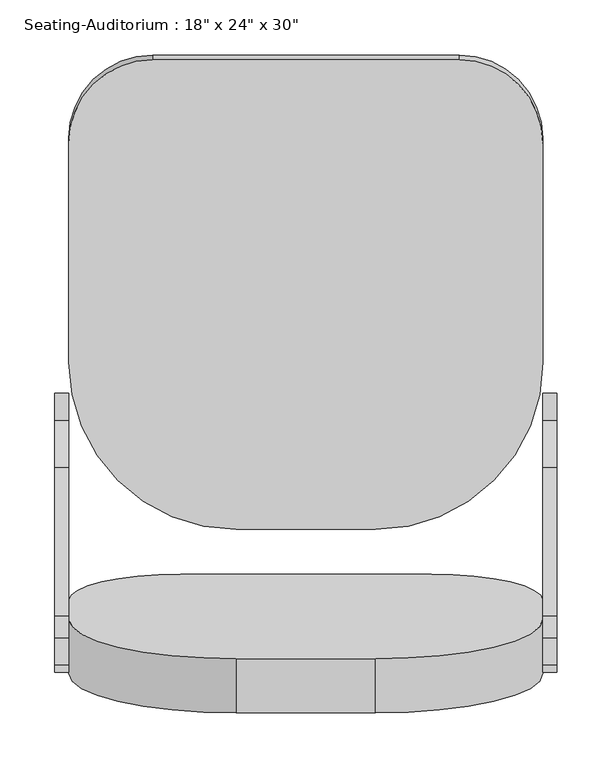
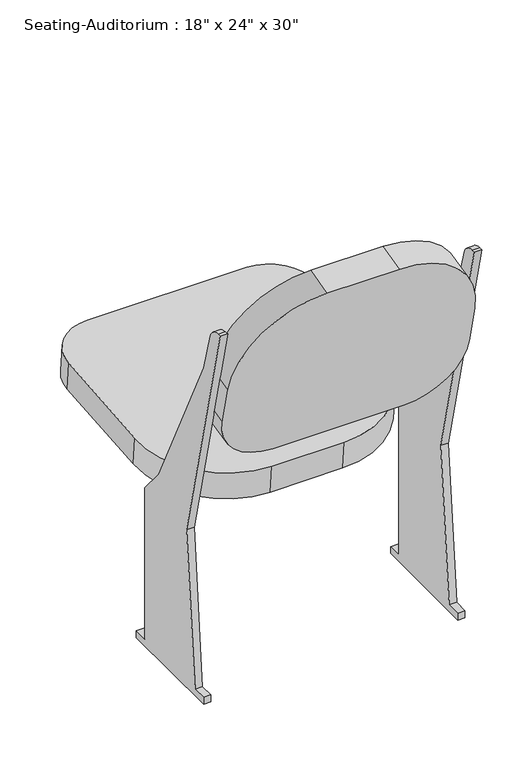
"""IFC4 building model written with IfcOpenShell, lengths in millimetres: furniture geometry."""

from ifc_helpers import new_model, si_unit, point, frame, frame_2d, origin, place, context, project, spatial, polyline, circle_curve, trimmed, segment, composite_curve, outline, extrude, source, transform, mapped, element, save


def furniture_eb3a3c23(model_context):
    return source(origin(), model_context, "Body", "SweptSolid", [
        extrude(outline(composite_curve([segment(polyline([(-13.3245902, 12.7), (12.0754098, 12.7), (37.4754098, 292.1), (-64.1245902, 711.2), (-57.883846, 711.2)]), True, "CONTINUOUS"), segment(trimmed(circle_curve(frame_2d((-57.883846, 685.8)), 25.4), [point((-57.883846, 711.2))], [point((-33.4611378, 692.7779166))], False, "CARTESIAN"), True, "CONTINUOUS"), segment(polyline([(-33.4611378, 692.7779166), (-13.3245902, 622.3), (121.8491486, 342.9), (164.4754098, 292.1), (164.4754098, 12.7), (189.8754098, 12.7), (189.8754098, 0.0), (-13.3245902, 0.0), (-13.3245902, 12.7)]), True, "CONTINUOUS")], self_intersect=False)), frame((376.6278689, 0.0, 0.0), z_axis=(1.0, 0.0, 0.0), x_axis=(0.0, 1.0, 0.0)), (0.0, 0.0, 1.0), 12.7),
        extrude(outline(composite_curve([segment(polyline([(-13.3245902, 0.0), (-13.3245902, 12.7), (12.0754098, 12.7), (37.4754098, 292.1), (-64.1245902, 711.2), (-57.883846, 711.2)]), True, "CONTINUOUS"), segment(trimmed(circle_curve(frame_2d((-57.883846, 685.8)), 25.4), [point((-57.883846, 711.2))], [point((-33.4611378, 692.7779166))], False, "CARTESIAN"), True, "CONTINUOUS"), segment(polyline([(-33.4611378, 692.7779166), (-13.3245902, 622.3), (121.8491486, 342.9), (164.4754098, 292.1), (164.4754098, 12.7), (189.8754098, 12.7), (189.8754098, 0.0), (-13.3245902, 0.0)]), True, "CONTINUOUS")], self_intersect=False)), frame((-67.8721311, 0.0, 0.0), z_axis=(1.0, 0.0, 0.0), x_axis=(0.0, 1.0, 0.0)), (0.0, 0.0, 1.0), 12.7),
        extrude(outline(composite_curve([segment(trimmed(circle_curve(frame_2d((0.0, -76.2)), 76.2), [point((0.0, 0.0))], [point((76.2, -76.2))], False, "CARTESIAN"), True, "CONTINUOUS"), segment(polyline([(76.2, -76.2), (76.2, -276.4123505)]), True, "CONTINUOUS"), segment(trimmed(circle_curve(frame_2d((-76.2, -276.4123505)), 152.4), [point((76.2, -276.4123505))], [point((-76.2, -428.8123506))], False, "CARTESIAN"), True, "CONTINUOUS"), segment(polyline([(-76.2, -428.8123506), (-203.2, -428.8123506)]), True, "CONTINUOUS"), segment(trimmed(circle_curve(frame_2d((-203.2, -276.4123505)), 152.4), [point((-203.2, -428.8123506))], [point((-355.6, -276.4123505))], False, "CARTESIAN"), True, "CONTINUOUS"), segment(polyline([(-355.6, -276.4123505), (-355.6, -76.2)]), True, "CONTINUOUS"), segment(trimmed(circle_curve(frame_2d((-279.4, -76.2)), 76.2), [point((-355.6, -76.2))], [point((-279.4, 0.0))], False, "CARTESIAN"), True, "CONTINUOUS"), segment(polyline([(-279.4, 0.0), (0.0, 0.0)]), True, "CONTINUOUS")], self_intersect=False)), frame((300.4278689, 497.5245173, 321.2380213), z_axis=(0.0, -0.08715574274765496, 0.9961946980917459), x_axis=(1.0, 0.0, 0.0)), (0.0, 0.0, 1.0), 50.8),
        extrude(outline(composite_curve([segment(polyline([(0.0, 0.0), (127.0, 0.0)]), True, "CONTINUOUS"), segment(trimmed(circle_curve(frame_2d((127.0, -152.4)), 152.4), [point((127.0, 0.0))], [point((279.4, -152.4))], False, "CARTESIAN"), True, "CONTINUOUS"), segment(polyline([(279.4, -152.4), (279.4, -224.0588601)]), True, "CONTINUOUS"), segment(trimmed(circle_curve(frame_2d((177.8, -224.0588601)), 101.6), [point((279.4, -224.0588601))], [point((177.8, -325.6588601))], False, "CARTESIAN"), True, "CONTINUOUS"), segment(polyline([(177.8, -325.6588601), (-50.8, -325.6588601)]), True, "CONTINUOUS"), segment(trimmed(circle_curve(frame_2d((-50.8, -224.0588601)), 101.6), [point((-50.8, -325.6588601))], [point((-152.4, -224.0588601))], False, "CARTESIAN"), True, "CONTINUOUS"), segment(polyline([(-152.4, -224.0588601), (-152.4, -152.4)]), True, "CONTINUOUS"), segment(trimmed(circle_curve(frame_2d((0.0, -152.4)), 152.4), [point((-152.4, -152.4))], [point((0.0, 0.0))], False, "CARTESIAN"), True, "CONTINUOUS")], self_intersect=False)), frame((224.2278689, -101.3396919, 755.9484479), z_axis=(0.0, 0.9717404775047361, 0.23605178325712217), x_axis=(-1.0, 0.0, 0.0)), (0.0, 0.0, 1.0), 50.8),
    ])


if __name__ == "__main__":
    model = new_model("IFC4")
    model_context = context("Model", 3, world=origin())
    ifc_project = project(units=[si_unit("LENGTHUNIT", "METRE", prefix="MILLI")], contexts=[model_context])
    site = spatial("IfcSite", under=ifc_project)
    building = spatial("IfcBuilding", under=site)
    placement = place(None, origin())
    furniture_shape = furniture_eb3a3c23(model_context)
    element("IfcFurniture", 1, ObjectType="Seating-Auditorium : 18\" x 24\" x 30\"", at=placement, inside=building, context=model_context, shape_type="MappedRepresentation", body=[
        mapped(furniture_shape, transform((0.0, 0.0, 0.0), x_axis=(1.0, 0.0, 0.0), y_axis=(0.0, 1.0, 0.0), z_axis=(0.0, 0.0, 1.0))),
    ])
    save(model, "model.ifc")

# Revit data of these elements
# Type "Seating-Auditorium : 18\" x 24\" x 30\""
#   Assembly Code = "E2020200"
#   Seat Material = Linen, Beige
#   Frame Material = Steel, Paint Finish, Dark Gray, Matte
#   Default Elevation = 0
# Element 1 (IfcFurniture, "Seating-Auditorium : 18\" x 24\" x 30\"")
#   Materials on its faces: "Steel, Paint Finish, Dark Gray, Matte", "Linen, Beige"
# Materials
#   "Linen, Beige": class "Textile", colour RGB 249 239 230, transparency 0, Description = "Linen, beige", Cost = 0
#   "Steel, Paint Finish, Dark Gray, Matte": class "Metal", colour RGB 98 98 98, transparency 0, Description = "Steel, paint finish, dark gray, matte", Cost = 0
